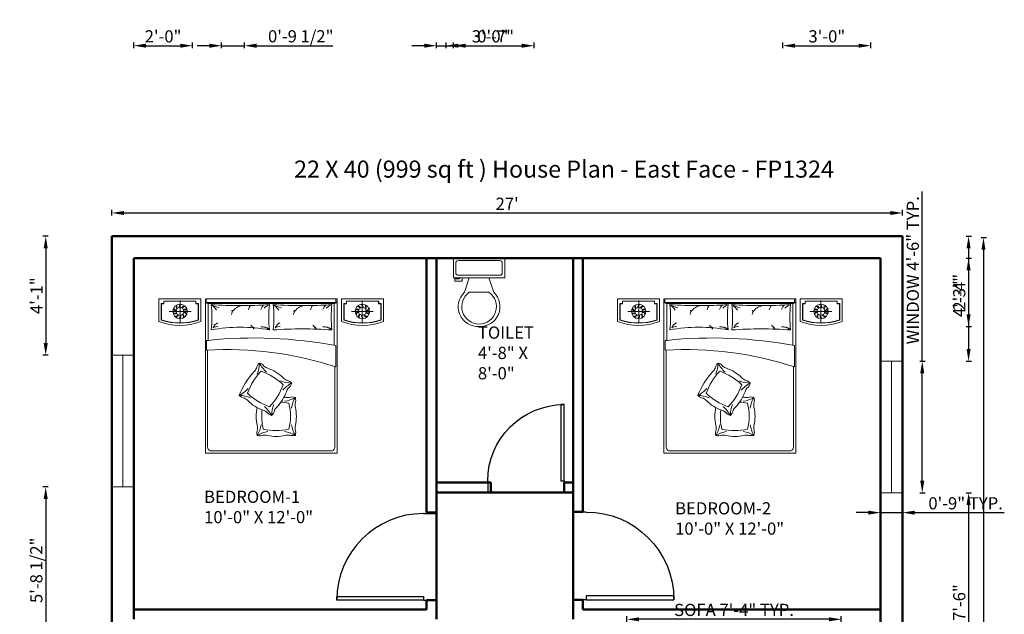
# Model space of a CAD drawing. Units: inches. Extents: x -8 to 396, y -471 to 106.
# Tile 4 of 4: x -8 to 396, y -138 to 106. Entities that reach past the tile are written whole.
import ezdxf

# ---------------------------------------------------------------- set-up
doc = ezdxf.new("R2010")
doc.units = ezdxf.units.IN
for name, color, linetype, lineweight in [('A-ANNO-DIMS', 2, 'Continuous', 18), ('A-ANNO-TEXT', 7, 'Continuous', 25), ('A-AREA-IDEN', 7, 'Continuous', 18), ('A-DOOR', 3, 'Continuous', 25), ('A-FLOR-FIXT', 9, 'Continuous', 18), ('A-GLAZ', 4, 'Continuous', 18), ('A-WALL', 7, 'Continuous', 50), ('furn', 8, 'Continuous', 18)]:
    doc.layers.add(name, color=color, linetype=linetype, lineweight=lineweight)
doc.styles.get("Standard").update_dxf_attribs({"font": 'arial.ttf'})
doc.dimstyles.new('ISO-25', dxfattribs={"dimtxt": 5, "dimasz": 5, "dimexe": 1.25, "dimexo": 0.625, "dimtad": 1, "dimlunit": 3, "dimtxsty": 'Standard', "dimcen": 2.5, "dimadec": 0, "dimazin": 0, "dimtfac": 1, "dimtmove": 0, "dimatfit": 3, "dimfxl": 1, "dimfxlon": 1, "dimarcsym": 0})

# ---------------------------------------------------------------- blocks, each defined once
blk = doc.blocks.new('*U7')
for p, q in [((9.5, -6), (9.5, -2)), ((-8, -8.5), (-8, -8)), ((-7, -8), (-7, -9.5)), ((-4, -8), (-6, -14)), ((4, -8), (6, -14)), ((-10, -8.5), (-8, -8.5)), ((-10, -9.5), (-10, -8.5)), ((-7, -9.5), (-10, -9.5)), ((4, -14), (-4, -14))]:
    blk.add_line(p, q)
blk.add_lwpolyline([(10.5, -8), (10.5, 0), (-10.5, 0), (-10.5, -8)], close=True)
for points in [[(-9.5, -2), (-9.5, -6)], [(8.5, -1), (-8.5, -1)], [(-8.5, -7), (8.5, -7)]]:
    blk.add_lwpolyline(points)
for centre, radius, start, end in [((-8.625, -1.875), 0.8839, 81.8699, 188.1301), ((8.625, -1.875), 0.8839, 351.8699, 98.1301), ((-8.625, -6.125), 0.8839, 171.869898, 278.1301), ((8.625, -6.125), 0.8839, 261.8699, 8.1301), ((-0.4772, -19.9188), 8.0953, 133.01722, 273.38), ((0.0374, -19.8731), 7.127, 124.50543, 269.7), ((-0.0373, -19.8731), 7.127, 270.3, 55.4946), ((0.4773, -19.9188), 8.0953, 266.62, 46.9828)]:
    blk.add_arc(centre, radius, start, end)
blk = doc.blocks.new('*U5')
for p, q in [((0, 0), (0, -6)), ((40, 0), (40, -6))]:
    blk.add_line(p, q)
blk.add_lwpolyline([(0, 0), (0, 40), (1.75, 40), (1.75, 0)], close=True)
blk.add_arc((0, 0), 40, 0, 90)
blk = doc.blocks.new('*D8')
at = {"layer": 'A-ANNO-DIMS', "color": 0, "lineweight": -2, "transparency": 16777216}
for p, q in [((29.97, 25.64), (29.97, 27.89)), ((34.97, 26.64), (348.97, 26.64)), ((353.97, 25.64), (353.97, 27.89))]:
    blk.add_line(p, q, dxfattribs=at)
at = {"layer": 'A-ANNO-DIMS', "color": 0, "transparency": 16777216}
for points in [[(34.97, 27.47), (34.97, 25.81), (29.97, 26.64)], [(348.97, 27.47), (348.97, 25.81), (353.97, 26.64)]]:
    blk.add_solid(points, dxfattribs=at)
at = {"layer": 'Defpoints', "color": 0, "transparency": 16777216}
for p in [(353.97, 26.64), (29.97, 16.55), (353.97, 16.55)]:
    blk.add_point(p, dxfattribs=at)
at = {"layer": 'A-ANNO-DIMS', "color": 0, "transparency": 16777216, "insert": (191.97, 29.78), "char_height": 5, "attachment_point": 5}
blk.add_mtext("27'", dxfattribs=at)
blk = doc.blocks.new('*D9')
at = {"layer": 'A-ANNO-DIMS', "color": 0, "lineweight": -2, "transparency": 16777216}
for p, q in [((386.16, 16.55), (388.41, 16.55)), ((387.16, 11.55), (387.16, -421.87)), ((386.16, -426.87), (388.41, -426.87))]:
    blk.add_line(p, q, dxfattribs=at)
at = {"layer": 'A-ANNO-DIMS', "color": 0, "transparency": 16777216}
for points in [[(386.32, 11.55), (387.99, 11.55), (387.16, 16.55)], [(386.32, -421.87), (387.99, -421.87), (387.16, -426.87)]]:
    blk.add_solid(points, dxfattribs=at)
at = {"layer": 'Defpoints', "color": 0, "transparency": 16777216}
for p in [(353.97, 16.55), (353.97, -426.87), (387.16, -426.87)]:
    blk.add_point(p, dxfattribs=at)
at = {"layer": 'A-ANNO-DIMS', "color": 0, "transparency": 16777216, "insert": (383.98, -205.16), "char_height": 5, "attachment_point": 5, "rotation": 90}
blk.add_mtext('36\'-11.43"', dxfattribs=at)
blk = doc.blocks.new('BED-DOUBLE-WITH-NIGHTSTANDS')
for p, q in [((8.67, 53.66), (8.67, 62.66)), ((19.97, 61.4), (72.06, 61.4)), ((20.23, 61.87), (20.23, 46.28)), ((71.76, 61.87), (71.76, 44.26)), ((83.36, 53.66), (83.36, 62.65)), ((4.17, 58.16), (13.17, 58.16)), ((87.86, 58.16), (78.86, 58.16))]:
    blk.add_line(p, q)
for points in [[(0, 53.96), (0, 63.32), (17.16, 63.32), (17.16, 53.96, -0.181818)], [(21.42, 50.55, 0.058596), (21.42, 60.97, 0.036889), (45.31, 60.97, 0.052163), (45.31, 50.55, 0.093111)], [(46.86, 50.55, 0.058596), (46.86, 60.97, 0.036648), (70.91, 60.97, 0.052163), (70.91, 50.55, 0.036967)], [(92.03, 53.97), (92.03, 63.33), (74.87, 63.33), (74.87, 53.97, 0.181818)], [(19.5, 46.28), (20.23, 46.28, -0.072944), (72.49, 44.11), (72.49, 35.45, 0.092568), (19.5, 42.31)]]:
    blk.add_lwpolyline(points, format="xyb", close=True)
for points in [[(1.97, 62.39), (1.97, 61.36), (0.94, 61.36)], [(2.06, 62.39), (2.06, 61.26), (0.94, 61.26)], [(1.97, 62.39), (15.19, 62.39)], [(1.97, 62.29), (15.19, 62.29)], [(15.1, 62.39), (15.1, 61.26), (16.22, 61.26)], [(15.19, 62.39), (15.19, 61.36), (16.22, 61.36)], [(19.03, 63.33), (19.03, 0), (73, 0), (73, 63.33)], [(72.49, 63.33), (72.49, 61.87), (19.34, 61.87), (19.34, 63.33), (73, 63.33)], [(76.84, 62.39), (76.84, 61.36), (75.81, 61.36)], [(76.93, 62.39), (76.93, 61.27), (75.81, 61.27)], [(90.06, 62.39), (76.84, 62.39)], [(90.06, 62.3), (76.84, 62.3)], [(89.97, 62.39), (89.97, 61.27), (91.09, 61.27)], [(90.06, 62.39), (90.06, 61.36), (91.09, 61.36)]]:
    blk.add_lwpolyline(points)
for points in [[(16.22, 61.36), (16.22, 54.62, -0.167087), (0.94, 54.62), (0.94, 61.36)], [(16.13, 61.36), (16.13, 54.68, -0.165559), (1.03, 54.68), (1.03, 61.36)], [(75.81, 61.36), (75.81, 54.62, 0.167087), (91.09, 54.62), (91.09, 61.36)], [(75.9, 61.36), (75.9, 54.69, 0.165559), (91, 54.69), (91, 61.36)], [(19.97, 42.34), (19.97, 2.5, 0.414214), (21.53, 0.94), (70.5, 0.94, 0.414214), (72.06, 2.5), (72.06, 35.61)], [(40.22, 32.4, 0.091296), (41.17, 36.97, 0.091296), (44.05, 33.3, 0.091296)], [(36.36, 24.6, 0.111006), (45.27, 19.06, 0.119549), (50.89, 28.07, 0.107813), (42, 33.64)], [(41.95, 33.62, 0.121865), (36.36, 24.6, 0.121865)], [(46.16, 15.49, 0.159461), (47.37, 17.63, -0.076283), (48.33, 18.96, 0.115075), (52.24, 25.25, -0.076283), (53.02, 26.7, 0.159461), (54.41, 28.73)], [(49.84, 29.69, 0.091296), (54.41, 28.73, 0.091296), (50.72, 25.86, 0.091296)], [(37.49, 22.77, 0.091296), (32.92, 23.74, 0.091296), (36.61, 26.6, 0.091296)], [(42.77, 9.86, 0.111006), (53.27, 9.87, 0.119549), (53.27, 20.49, 0.033212), (50.04, 20.98)], [(51.53, 21.31, 0.091296), (55.91, 22.91, 0.091296), (54.3, 18.53, 0.091296)], [(55.91, 7.31, 0.159461), (55.8, 9.77, -0.076283), (55.91, 11.41, 0.115075), (55.91, 18.81, -0.076283), (55.8, 20.45, 0.159461), (55.91, 22.91)], [(47.11, 20.06, 0.091296), (46.16, 15.49, 0.091296), (43.28, 19.16)], [(44.7, 8.91, 0.091296), (40.31, 7.31, 0.091296), (41.93, 11.69, 0.091296)], [(54.3, 11.69, 0.091296), (55.91, 7.31, 0.091296), (51.53, 8.91)]]:
    blk.add_lwpolyline(points, format="xyb")
for centre, radius in [((8.67, 58.16), 2.94), ((83.36, 58.16), 2.94), ((8.67, 58.16), 1.59), ((83.36, 58.16), 1.59)]:
    blk.add_circle(centre, radius)
for centre, radius, start, end in [((8.93, 60.36), 1.89, 172.17, 218.4897), ((8.74, 60.32), 1.44, 160.3002, 220.538), ((10.17, 59.78), 1.89, 136.17, 182.4897), ((10, 59.86), 1.44, 124.3002, 184.538), ((19.97, 62.34), 0.936, 180, 270), ((26.97, 69.69), 10.33, 237.5379, 257.5233), ((13.61, 51.22), 12.5, 36.4935, 51.2792), ((34.89, 54.79), 5.78, 96.6849, 148.3182), ((40.74, 58.08), 4.06, 141.8174, 169.8987), ((45.87, 57.5), 4.36, 130.5354, 160.3558), ((48.59, 53.82), 7.86, 114.6457, 134.1585), ((39.05, 51.22), 12.5, 36.4935, 51.2792), ((52.41, 69.69), 10.33, 237.5379, 257.5233), ((60.33, 54.79), 5.78, 96.6849, 148.3182), ((66.18, 58.08), 4.06, 141.8174, 169.8987), ((71.31, 57.5), 4.36, 130.5354, 160.3558), ((74.03, 53.82), 7.86, 114.6457, 134.1585), ((72.06, 62.34), 0.936, 270, 0), ((82.03, 59.86), 1.44, 355.462, 55.6998), ((81.86, 59.78), 1.89, 357.5103, 43.83), ((83.28, 60.32), 1.44, 319.462, 19.6998), ((83.31, 60.44), 1.89, 321.5103, 7.83), ((6.64, 58.9), 1.44, 232.3002, 292.538), ((6.65, 59.08), 1.89, 244.17, 290.4897), ((7.58, 60.09), 1.89, 208.17, 254.4897), ((7.46, 59.95), 1.44, 196.3002, 256.538), ((6.59, 57.56), 1.44, 268.3002, 328.538), ((6.49, 57.72), 1.89, 280.17, 326.4897), ((7.34, 56.45), 1.44, 304.3002, 4.538), ((7.16, 56.53), 1.89, 316.17, 2.4897), ((10.84, 58.59), 1.89, 100.17, 146.4897), ((10.75, 58.75), 1.44, 88.3002, 148.538), ((8.59, 56), 1.44, 340.3002, 40.538), ((8.41, 55.96), 1.89, 352.17, 38.4897), ((10.68, 57.23), 1.89, 64.17, 110.4897), ((10.7, 57.42), 1.44, 52.3002, 112.538), ((9.88, 56.36), 1.44, 16.3002, 76.538), ((9.75, 56.22), 1.89, 28.17, 74.4897), ((27.39, 58.01), 2.59, 335.8927, 16.1192), ((52.83, 58.01), 2.59, 335.8927, 16.1192), ((81.33, 57.42), 1.44, 67.462, 127.6998), ((81.35, 57.23), 1.89, 69.5103, 115.83), ((82.28, 56.22), 1.89, 105.5103, 151.83), ((82.15, 56.36), 1.44, 103.462, 163.6998), ((81.28, 58.75), 1.44, 31.462, 91.6998), ((81.19, 58.59), 1.89, 33.5103, 79.83), ((83.62, 55.95), 1.89, 141.5103, 187.83), ((83.44, 56), 1.44, 139.462, 199.6998), ((84.86, 56.53), 1.89, 177.5103, 223.83), ((84.69, 56.45), 1.44, 175.462, 235.6998), ((85.53, 57.72), 1.89, 213.5103, 259.83), ((85.44, 57.56), 1.44, 211.462, 271.6998), ((85.59, 59.16), 1.89, 249.5103, 295.83), ((85.61, 58.98), 1.44, 247.462, 307.6998), ((84.78, 60.03), 1.44, 283.462, 343.6998), ((84.66, 60.17), 1.89, 285.5103, 331.83), ((25.53, 50.31), 3.47, 114.2916, 160.9896), ((28.45, 43.29), 13.02, 36.2085, 45.0849), ((50.97, 50.31), 3.47, 114.2916, 160.9896), ((53.89, 43.29), 13.02, 36.2085, 45.0849), ((23.73, 49.58), 2.37, 76.4823, 128.5563), ((38.09, 50.99), 0.874, 353.7543, 77.2187), ((42.26, 47.56), 4.26, 44.406, 96.8342), ((43.06, 49.05), 2.7, 33.6349, 90.8456), ((49.17, 49.58), 2.37, 76.4823, 128.5563), ((63.53, 50.99), 0.874, 353.7543, 77.2187), ((67.7, 47.56), 4.26, 44.406, 96.8342), ((68.5, 49.05), 2.7, 33.6349, 90.8456), ((43.84, 34.06), 3.95, 132.4658, 168.7065), ((40.13, 33.31), 3.82, 37.2937, 74.0973), ((64.54, 10.81), 34.16, 138.3818, 157.7644), ((35.14, 37.29), 5.42, 315.5854, 333.0343), ((46.4, 39.96), 5.42, 233.2983, 250.7472), ((39.41, 19.4), 16.3, 45.1307, 71.3884), ((54.69, 34.83), 5.42, 225.7718, 243.2208), ((51.59, 26.4), 3.65, 39.4726, 79.6505), ((35.83, 26.42), 3.95, 222.6522, 258.8929), ((32.63, 17.7), 5.42, 45.7718, 63.2208), ((47.9, 33.13), 16.3, 225.1307, 251.3884), ((48.11, 7.06), 16.3, 77.0576, 78.7033), ((52.92, 28.24), 5.42, 257.6988, 275.1477), ((54.75, 19.45), 3.65, 71.3996, 111.5774), ((56.19, 15.11), 16.3, 166.8711, 193.1289), ((64.23, 15.22), 22.11, 173.1956, 194.0284), ((40.92, 12.57), 5.42, 53.2983, 70.7472), ((47.68, 19.75), 4.52, 218.7754, 250.3571), ((44.12, 8.37), 3.95, 159.3666, 195.6073), ((35.03, 10.24), 5.42, 355.0387, 12.4877), ((41.36, 11.12), 3.95, 254.5791, 290.8198), ((43.26, 2.03), 5.42, 77.6988, 95.1477), ((48.06, 23.21), 16.3, 257.0576, 283.3153), ((53, 2.06), 5.42, 85.2252, 102.6741), ((54.95, 11.73), 4.52, 250.7023, 282.284)]:
    blk.add_arc(centre, radius, start, end)
blk = doc.blocks.new('WINDOW-54IN')
blk.add_line((4.5, 54), (4.5, 0))
blk.add_lwpolyline([(0, 54), (9, 54), (9, 0), (0, 0)], close=True)
blk = doc.blocks.new('*D14')
at = {"layer": 'A-ANNO-DIMS', "color": 0, "lineweight": -2, "transparency": 16777216}
for p, q in [((362.07, -34.09), (362.07, 35.43)), ((361.07, -34.09), (363.32, -34.09)), ((362.07, -83.09), (362.07, -39.09)), ((361.07, -88.09), (363.32, -88.09))]:
    blk.add_line(p, q, dxfattribs=at)
at = {"layer": 'A-ANNO-DIMS', "color": 0, "transparency": 16777216}
for points in [[(361.23, -39.09), (362.9, -39.09), (362.07, -34.09)], [(361.23, -83.09), (362.9, -83.09), (362.07, -88.09)]]:
    blk.add_solid(points, dxfattribs=at)
at = {"layer": 'Defpoints', "color": 0, "transparency": 16777216}
for p in [(353.97, -34.09), (362.07, -34.09), (353.97, -88.09)]:
    blk.add_point(p, dxfattribs=at)
at = {"layer": 'A-ANNO-DIMS', "color": 0, "transparency": 16777216, "insert": (358.85, 3.17), "char_height": 5, "attachment_point": 5, "rotation": 90}
blk.add_mtext('WINDOW 4\'-6" TYP.', dxfattribs=at)
blk = doc.blocks.new('*D15')
at = {"layer": 'A-ANNO-DIMS', "color": 0, "lineweight": -2, "transparency": 16777216}
for p, q in [((339.97, -96.19), (334.97, -96.19)), ((344.97, -95.19), (344.97, -97.44)), ((344.97, -96.19), (353.97, -96.19)), ((353.97, -95.19), (353.97, -97.44)), ((358.97, -96.19), (395.69, -96.19))]:
    blk.add_line(p, q, dxfattribs=at)
at = {"layer": 'A-ANNO-DIMS', "color": 0, "transparency": 16777216}
for points in [[(339.97, -95.36), (339.97, -97.02), (344.97, -96.19)], [(358.97, -95.36), (358.97, -97.02), (353.97, -96.19)]]:
    blk.add_solid(points, dxfattribs=at)
at = {"layer": 'Defpoints', "color": 0, "transparency": 16777216}
for p in [(344.97, -88.09), (353.97, -88.09), (353.97, -96.19)]:
    blk.add_point(p, dxfattribs=at)
at = {"layer": 'A-ANNO-DIMS', "color": 0, "transparency": 16777216, "insert": (379.83, -93.01), "char_height": 5, "attachment_point": 5}
blk.add_mtext('0\'-9" TYP.', dxfattribs=at)
blk = doc.blocks.new('*D18')
at = {"layer": 'A-ANNO-DIMS', "color": 0, "lineweight": -2, "transparency": 16777216}
for p, q in [((241.05, -140.93), (241.05, -138.68)), ((323.86, -139.93), (246.05, -139.93)), ((328.86, -140.93), (328.86, -138.68))]:
    blk.add_line(p, q, dxfattribs=at)
at = {"layer": 'A-ANNO-DIMS', "color": 0, "transparency": 16777216}
for points in [[(246.05, -139.1), (246.05, -140.76), (241.05, -139.93)], [(323.86, -139.1), (323.86, -140.76), (328.86, -139.93)]]:
    blk.add_solid(points, dxfattribs=at)
at = {"layer": 'Defpoints', "color": 0, "transparency": 16777216}
for p in [(241.05, -139.93), (241.05, -153.1), (328.86, -153.1)]:
    blk.add_point(p, dxfattribs=at)
at = {"layer": 'A-ANNO-DIMS', "color": 0, "transparency": 16777216, "insert": (284.95, -136.72), "char_height": 5, "attachment_point": 5}
blk.add_mtext('SOFA 7\'-4" TYP.', dxfattribs=at)
blk = doc.blocks.new('*D28')
at = {"layer": 'A-ANNO-DIMS', "color": 0, "lineweight": -2, "transparency": 16777216}
for p, q in [((3.88, 17.13), (1.63, 17.13)), ((2.88, 12.13), (2.88, -26.66)), ((3.88, -31.66), (1.63, -31.66))]:
    blk.add_line(p, q, dxfattribs=at)
at = {"layer": 'A-ANNO-DIMS', "color": 0, "transparency": 16777216}
for points in [[(2.04, 12.13), (3.71, 12.13), (2.88, 17.13)], [(2.04, -26.66), (3.71, -26.66), (2.88, -31.66)]]:
    blk.add_solid(points, dxfattribs=at)
at = {"layer": 'Defpoints', "color": 0, "transparency": 16777216}
for p in [(29.97, 17.13), (2.88, -31.66), (29.97, -31.66)]:
    blk.add_point(p, dxfattribs=at)
at = {"layer": 'A-ANNO-DIMS', "color": 0, "transparency": 16777216, "insert": (-0.26, -7.27), "char_height": 5, "attachment_point": 5, "rotation": 90}
blk.add_mtext('4\'-1"', dxfattribs=at)
blk = doc.blocks.new('*D29')
at = {"layer": 'A-ANNO-DIMS', "color": 0, "lineweight": -2, "transparency": 16777216}
for p, q in [((3.88, -85.66), (1.63, -85.66)), ((2.88, -90.66), (2.88, -149)), ((3.88, -154), (1.63, -154))]:
    blk.add_line(p, q, dxfattribs=at)
at = {"layer": 'A-ANNO-DIMS', "color": 0, "transparency": 16777216}
for points in [[(2.04, -90.66), (3.71, -90.66), (2.88, -85.66)], [(2.04, -149), (3.71, -149), (2.88, -154)]]:
    blk.add_solid(points, dxfattribs=at)
at = {"layer": 'Defpoints', "color": 0, "transparency": 16777216}
for p in [(29.97, -85.66), (2.88, -154), (29.97, -154)]:
    blk.add_point(p, dxfattribs=at)
at = {"layer": 'A-ANNO-DIMS', "color": 0, "transparency": 16777216, "insert": (-0.33, -119.83), "char_height": 5, "attachment_point": 5, "rotation": 90}
blk.add_mtext('5\'-8 1/2"', dxfattribs=at)
blk = doc.blocks.new('*D31')
at = {"layer": 'A-ANNO-DIMS', "color": 0, "lineweight": -2, "transparency": 16777216}
for p, q in [((380.06, 17.13), (382.31, 17.13)), ((381.06, 12.13), (381.06, -29.09)), ((380.06, -34.09), (382.31, -34.09))]:
    blk.add_line(p, q, dxfattribs=at)
at = {"layer": 'A-ANNO-DIMS', "color": 0, "transparency": 16777216}
for points in [[(380.22, 12.13), (381.89, 12.13), (381.06, 17.13)], [(380.22, -29.09), (381.89, -29.09), (381.06, -34.09)]]:
    blk.add_solid(points, dxfattribs=at)
at = {"layer": 'Defpoints', "color": 0, "transparency": 16777216}
for p in [(353.97, 17.13), (353.97, -34.09), (381.06, -34.09)]:
    blk.add_point(p, dxfattribs=at)
at = {"layer": 'A-ANNO-DIMS', "color": 0, "transparency": 16777216, "insert": (377.88, -8.48), "char_height": 5, "attachment_point": 5, "rotation": 90}
blk.add_mtext('4\'-3"', dxfattribs=at)
blk = doc.blocks.new('*D32')
at = {"layer": 'A-ANNO-DIMS', "color": 0, "lineweight": -2, "transparency": 16777216}
for p, q in [((380.06, -88.09), (382.31, -88.09)), ((381.06, -93.09), (381.06, -173.04)), ((380.06, -178.04), (382.31, -178.04))]:
    blk.add_line(p, q, dxfattribs=at)
at = {"layer": 'A-ANNO-DIMS', "color": 0, "transparency": 16777216}
for points in [[(380.22, -93.09), (381.89, -93.09), (381.06, -88.09)], [(380.22, -173.04), (381.89, -173.04), (381.06, -178.04)]]:
    blk.add_solid(points, dxfattribs=at)
at = {"layer": 'Defpoints', "color": 0, "transparency": 16777216}
for p in [(353.97, -88.09), (353.97, -178.04), (381.06, -178.04)]:
    blk.add_point(p, dxfattribs=at)
at = {"layer": 'A-ANNO-DIMS', "color": 0, "transparency": 16777216, "insert": (377.88, -133.06), "char_height": 5, "attachment_point": 5, "rotation": 90}
blk.add_mtext('7\'-6"', dxfattribs=at)
blk = doc.blocks.new('*D39')
at = {"layer": 'A-ANNO-DIMS', "color": 0, "lineweight": -2, "transparency": 16777216}
for p, q in [((69.97, 95.22), (64.97, 95.22)), ((74.97, 94.22), (74.97, 96.47)), ((74.97, 95.22), (84.3, 95.22)), ((84.3, 94.22), (84.3, 96.47)), ((89.3, 95.22), (120.49, 95.22))]:
    blk.add_line(p, q, dxfattribs=at)
at = {"layer": 'A-ANNO-DIMS', "color": 0, "transparency": 16777216}
for points in [[(69.97, 96.05), (69.97, 94.38), (74.97, 95.22)], [(89.3, 96.05), (89.3, 94.38), (84.3, 95.22)]]:
    blk.add_solid(points, dxfattribs=at)
at = {"layer": 'Defpoints', "color": 0, "transparency": 16777216}
for p in [(84.3, 95.22), (74.97, -139.87), (84.3, -139.87)]:
    blk.add_point(p, dxfattribs=at)
at = {"layer": 'A-ANNO-DIMS', "color": 0, "transparency": 16777216, "insert": (107.39, 98.43), "char_height": 5, "attachment_point": 5}
blk.add_mtext('0\'-9 1/2"', dxfattribs=at)
blk = doc.blocks.new('*D40')
at = {"layer": 'A-ANNO-DIMS', "color": 0, "lineweight": -2, "transparency": 16777216}
for p, q in [((38.97, 94.22), (38.97, 96.47)), ((43.97, 95.22), (57.97, 95.22)), ((62.97, 94.22), (62.97, 96.47))]:
    blk.add_line(p, q, dxfattribs=at)
at = {"layer": 'A-ANNO-DIMS', "color": 0, "transparency": 16777216}
for points in [[(43.97, 96.05), (43.97, 94.38), (38.97, 95.22)], [(57.97, 96.05), (57.97, 94.38), (62.97, 95.22)]]:
    blk.add_solid(points, dxfattribs=at)
at = {"layer": 'Defpoints', "color": 0, "transparency": 16777216}
for p in [(62.97, 95.22), (38.97, -303.72), (62.97, -303.72)]:
    blk.add_point(p, dxfattribs=at)
at = {"layer": 'A-ANNO-DIMS', "color": 0, "transparency": 16777216, "insert": (50.97, 98.39), "char_height": 5, "attachment_point": 5}
blk.add_mtext('2\'-0"', dxfattribs=at)
blk = doc.blocks.new('*D46')
at = {"layer": 'A-ANNO-DIMS', "color": 0, "lineweight": -2, "transparency": 16777216}
for p, q in [((185.28, -452.96), (185.28, -455.21)), ((190.28, -453.96), (210.28, -453.96)), ((215.28, -452.96), (215.28, -455.21))]:
    blk.add_line(p, q, dxfattribs=at)
at = {"layer": 'A-ANNO-DIMS', "color": 0, "transparency": 16777216}
for points in [[(190.28, -453.13), (190.28, -454.8), (185.28, -453.96)], [(210.28, -453.13), (210.28, -454.8), (215.28, -453.96)]]:
    blk.add_solid(points, dxfattribs=at)
at = {"layer": 'Defpoints', "color": 0, "transparency": 16777216}
for p in [(185.28, -87.87), (215.28, -87.87), (215.28, -453.96)]:
    blk.add_point(p, dxfattribs=at)
at = {"layer": 'A-ANNO-DIMS', "color": 0, "transparency": 16777216, "insert": (200.28, -450.79), "char_height": 5, "attachment_point": 5}
blk.add_mtext('2\'-6"', dxfattribs=at)
blk = doc.blocks.new('*D47')
at = {"layer": 'A-ANNO-DIMS', "color": 0, "lineweight": -2, "transparency": 16777216}
for p, q in [((157.97, 95.22), (152.97, 95.22)), ((162.97, 94.22), (162.97, 96.47)), ((162.97, 95.22), (169.97, 95.22)), ((169.97, 94.22), (169.97, 96.47)), ((174.97, 95.22), (194.51, 95.22))]:
    blk.add_line(p, q, dxfattribs=at)
at = {"layer": 'A-ANNO-DIMS', "color": 0, "transparency": 16777216}
for points in [[(157.97, 96.05), (157.97, 94.38), (162.97, 95.22)], [(174.97, 96.05), (174.97, 94.38), (169.97, 95.22)]]:
    blk.add_solid(points, dxfattribs=at)
at = {"layer": 'Defpoints', "color": 0, "transparency": 16777216}
for p in [(169.97, 95.22), (162.97, 8.13), (169.97, 8.13)]:
    blk.add_point(p, dxfattribs=at)
at = {"layer": 'A-ANNO-DIMS', "color": 0, "transparency": 16777216, "insert": (187.24, 98.39), "char_height": 5, "attachment_point": 5}
blk.add_mtext('0\'-7"', dxfattribs=at)
blk = doc.blocks.new('*D48')
at = {"layer": 'A-ANNO-DIMS', "color": 0, "lineweight": -2, "transparency": 16777216}
for p, q in [((169.97, -452.96), (169.97, -455.21)), ((174.97, -453.96), (185.97, -453.96)), ((190.97, -452.96), (190.97, -455.21))]:
    blk.add_line(p, q, dxfattribs=at)
at = {"layer": 'A-ANNO-DIMS', "color": 0, "transparency": 16777216}
for points in [[(174.97, -453.13), (174.97, -454.8), (169.97, -453.96)], [(185.97, -453.13), (185.97, -454.8), (190.97, -453.96)]]:
    blk.add_solid(points, dxfattribs=at)
at = {"layer": 'Defpoints', "color": 0, "transparency": 16777216}
for p in [(169.97, 0.13), (190.97, 0.13), (190.97, -453.96)]:
    blk.add_point(p, dxfattribs=at)
at = {"layer": 'A-ANNO-DIMS', "color": 0, "transparency": 16777216, "insert": (180.47, -450.79), "char_height": 5, "attachment_point": 5}
blk.add_mtext('1\'-9"', dxfattribs=at)
blk = doc.blocks.new('*D49')
at = {"layer": 'A-ANNO-DIMS', "color": 0, "lineweight": -2, "transparency": 16777216}
for p, q in [((380.06, 8.13), (382.31, 8.13)), ((381.06, 3.13), (381.06, -14.87)), ((380.06, -19.87), (382.31, -19.87))]:
    blk.add_line(p, q, dxfattribs=at)
at = {"layer": 'A-ANNO-DIMS', "color": 0, "transparency": 16777216}
for points in [[(380.22, 3.13), (381.89, 3.13), (381.06, 8.13)], [(380.22, -14.87), (381.89, -14.87), (381.06, -19.87)]]:
    blk.add_solid(points, dxfattribs=at)
at = {"layer": 'Defpoints', "color": 0, "transparency": 16777216}
for p in [(190.97, 8.13), (180.47, -19.87), (381.06, -19.87)]:
    blk.add_point(p, dxfattribs=at)
at = {"layer": 'A-ANNO-DIMS', "color": 0, "transparency": 16777216, "insert": (377.92, -5.87), "char_height": 5, "attachment_point": 5, "rotation": 90}
blk.add_mtext('2\'-4"', dxfattribs=at)
blk = doc.blocks.new('*D50')
at = {"layer": 'A-ANNO-DIMS', "color": 0, "lineweight": -2, "transparency": 16777216}
for p, q in [((166.97, 94.22), (166.97, 96.47)), ((171.97, 95.22), (197.97, 95.22)), ((202.97, 94.22), (202.97, 96.47))]:
    blk.add_line(p, q, dxfattribs=at)
at = {"layer": 'A-ANNO-DIMS', "color": 0, "transparency": 16777216}
for points in [[(171.97, 96.05), (171.97, 94.38), (166.97, 95.22)], [(197.97, 96.05), (197.97, 94.38), (202.97, 95.22)]]:
    blk.add_solid(points, dxfattribs=at)
at = {"layer": 'Defpoints', "color": 0, "transparency": 16777216}
for p in [(202.97, 95.22), (166.97, -317.87), (202.97, -317.87)]:
    blk.add_point(p, dxfattribs=at)
at = {"layer": 'A-ANNO-DIMS', "color": 0, "transparency": 16777216, "insert": (184.97, 98.4), "char_height": 5, "attachment_point": 5}
blk.add_mtext('3\'-0"', dxfattribs=at)
blk = doc.blocks.new('*D52')
at = {"layer": 'A-ANNO-DIMS', "color": 0, "lineweight": -2, "transparency": 16777216}
for p, q in [((304.97, 94.22), (304.97, 96.47)), ((309.97, 95.22), (335.97, 95.22)), ((340.97, 94.22), (340.97, 96.47))]:
    blk.add_line(p, q, dxfattribs=at)
at = {"layer": 'A-ANNO-DIMS', "color": 0, "transparency": 16777216}
for points in [[(309.97, 96.05), (309.97, 94.38), (304.97, 95.22)], [(335.97, 96.05), (335.97, 94.38), (340.97, 95.22)]]:
    blk.add_solid(points, dxfattribs=at)
at = {"layer": 'Defpoints', "color": 0, "transparency": 16777216}
for p in [(340.97, 95.22), (304.97, -293.87), (340.97, -293.87)]:
    blk.add_point(p, dxfattribs=at)
at = {"layer": 'A-ANNO-DIMS', "color": 0, "transparency": 16777216, "insert": (322.97, 98.4), "char_height": 5, "attachment_point": 5}
blk.add_mtext('3\'-0"', dxfattribs=at)

msp = doc.modelspace()

# ---------------------------------------------------------------- linework, layer by layer
at = {"layer": 'A-WALL'}
for p, q in [((29.966, 17.126), (353.966, 17.126)), ((29.966, -426.874), (29.966, 17.126)), ((353.966, 17.126), (353.966, -426.874)), ((38.966, 8.126), (162.966, 8.126)), ((38.966, -139.874), (38.966, 8.126)), ((158.966, -96.08), (158.966, 8.126)), ((162.966, 8.126), (218.966, 8.126)), ((162.966, -139.874), (162.966, 8.126)), ((218.966, 8.126), (344.966, 8.126)), ((218.966, -139.874), (218.966, 8.126)), ((222.966, -95.874), (222.966, 8.126)), ((344.966, 8.126), (344.966, -417.874)), ((162.966, -83.874), (185.282, -83.874)), ((185.282, -83.874), (185.282, -87.874)), ((215.282, -83.874), (215.282, -87.874)), ((215.282, -83.874), (218.966, -83.874)), ((162.966, -87.874), (218.966, -87.874)), ((158.966, -96.08), (162.966, -96.08)), ((222.966, -95.874), (218.966, -95.874)), ((158.966, -132.08), (162.966, -132.08)), ((158.966, -135.874), (158.966, -132.08)), ((222.966, -131.874), (218.966, -131.874)), ((222.966, -135.874), (222.966, -131.874)), ((38.966, -135.874), (158.966, -135.874)), ((222.966, -135.874), (344.966, -135.874))]:
    msp.add_line(p, q, dxfattribs=at)

# ---------------------------------------------------------------- block references
at = {"layer": 'A-DOOR', "xscale": -0.7819833272519193, "yscale": 0.7819833272519193, "zscale": 0.7819833272519193}
msp.add_blockref('*U5', (215.282, -83.182), dxfattribs=at)
at = {"layer": 'A-DOOR'}
for p, xscale, yscale, zscale, rotation in [((157.639, -132.08), 0.8877503757117265, 0.8877503757117265, 0.8877503757117265, 90), ((224.356, -131.874), -0.8984837037046304, 0.8984837037046304, 0.8984837037046304, 270)]:
    msp.add_blockref('*U5', p, dxfattribs=dict(at, xscale=xscale, yscale=yscale, zscale=zscale, rotation=rotation))
at = {"layer": 'A-FLOR-FIXT'}
msp.add_blockref('*U7', (180.466, 8.126), dxfattribs=at)
at = {"layer": 'A-GLAZ'}
for p in [(29.966, -85.659), (344.966, -88.091)]:
    msp.add_blockref('WINDOW-54IN', p, dxfattribs=at)
at = {"layer": 'furn'}
for p in [(49.255, -71.857), (237.207, -71.857)]:
    msp.add_blockref('BED-DOUBLE-WITH-NIGHTSTANDS', p, dxfattribs=at)

# ---------------------------------------------------------------- texts
at = {"layer": 'A-ANNO-TEXT', "insert": (104.662, 48.134), "char_height": 7, "attachment_point": 1}
msp.add_mtext_dynamic_manual_height_columns('22 X 40 (999 sq ft ) House Plan - East Face - FP1324', width=277.00832, gutter_width=12.5, heights=[0], dxfattribs=at)
at = {"layer": 'A-AREA-IDEN', "char_height": 5, "attachment_point": 1}
for s, width, insert in [('TOILET\\P4\'-8" X 8\'-0"', 33.92558, (179.988, -19.888)), ('BEDROOM-1\\P10\'-0" X 12\'-0"', 67.54976, (67.779, -87.2)), ('BEDROOM-2\\P10\'-0" X 12\'-0"', 62.93055, (260.798, -91.915))]:
    msp.add_mtext_dynamic_manual_height_columns(s, width=width, gutter_width=12.5, heights=[0], dxfattribs=dict(at, insert=insert))

# ---------------------------------------------------------------- dimensions: what is measured, and where the dimension line sits
at = {"layer": 'A-ANNO-DIMS'}
for base, p1, p2, override, picture, middle in [((84.299, 95.216), (74.966, -139.874), (84.299, -139.874), {"dimdec": 1, "dimlfac": 1, "dimrnd": 0, "dimzin": 1, "dimdsep": 46, "dimlunit": 4, "dimfrac": 2}, '*D39', (107.395, 98.426)), ((62.966, 95.216), (38.966, -303.723), (62.966, -303.723), {"dimdec": 1, "dimlfac": 1, "dimrnd": 0, "dimzin": 1, "dimdsep": 46, "dimlunit": 4, "dimfrac": 2}, '*D40', (50.966, 98.394)), ((169.966, 95.216), (162.966, 8.126), (169.966, 8.126), {"dimdec": 1, "dimlfac": 1, "dimrnd": 0, "dimzin": 1, "dimdsep": 46, "dimlunit": 4, "dimfrac": 2}, '*D47', (187.236, 98.394)), ((202.966, 95.216), (166.966, -317.874), (202.966, -317.874), {"dimdec": 1, "dimlfac": 1, "dimrnd": 0, "dimzin": 1, "dimdsep": 46, "dimlunit": 4, "dimfrac": 2}, '*D50', (184.966, 98.396)), ((340.966, 95.216), (304.966, -293.874), (340.966, -293.874), {"dimdec": 1, "dimlfac": 1, "dimrnd": 0, "dimzin": 1, "dimdsep": 46, "dimlunit": 4, "dimfrac": 2}, '*D52', (322.966, 98.396)), ((353.966, 26.64), (29.966, 16.551), (353.966, 16.551), {"dimclrd": 0, "dimclre": 0, "dimclrt": 0}, '*D8', (191.966, 29.775)), ((190.966, -453.964), (169.966, 0.126), (190.966, 0.126), {"dimdec": 1, "dimlfac": 1, "dimrnd": 0, "dimzin": 1, "dimdsep": 46, "dimlunit": 4, "dimfrac": 2}, '*D48', (180.466, -450.786)), ((215.282, -453.964), (185.282, -87.874), (215.282, -87.874), {"dimdec": 1, "dimlfac": 1, "dimrnd": 0, "dimzin": 1, "dimdsep": 46, "dimlunit": 4, "dimfrac": 2}, '*D46', (200.282, -450.786))]:
    dim = msp.add_linear_dim(base=base, p1=p1, p2=p2, dimstyle='ISO-25', override=override, dxfattribs=at)
    dim.commit()
    dim.dimension.update_dxf_attribs({"geometry": picture, "text_midpoint": middle})
for base, p1, p2, angle, text, picture, middle in [((362.066, -34.09), (353.966, -88.09), (353.966, -34.09), 90, 'WINDOW <> TYP.', '*D14', (358.854, 3.17)), ((241.049, -139.93), (328.86, -153.102), (241.049, -153.102), 180, 'SOFA <> TYP.', '*D18', (284.954, -136.718))]:
    dim = msp.add_linear_dim(base=base, p1=p1, p2=p2, angle=angle, text=text, dimstyle='ISO-25', override={"dimdec": 1, "dimlfac": 1, "dimrnd": 0, "dimzin": 1, "dimdsep": 46, "dimlunit": 4, "dimfrac": 2}, dxfattribs=at)
    dim.commit()
    dim.dimension.update_dxf_attribs({"geometry": picture, "text_midpoint": middle})
for base, p1, p2, override, picture, middle in [((2.876, -31.659), (29.966, 17.126), (29.966, -31.659), {"dimdec": 1, "dimlfac": 1, "dimrnd": 0, "dimzin": 1, "dimdsep": 46, "dimlunit": 4, "dimfrac": 2}, '*D28', (-0.26, -7.266)), ((381.056, -34.09), (353.966, 17.126), (353.966, -34.09), {"dimdec": 1, "dimlfac": 1, "dimrnd": 0, "dimzin": 1, "dimdsep": 46, "dimlunit": 4, "dimfrac": 2}, '*D31', (377.876, -8.482)), ((387.1551, -426.874), (353.9656, 16.5511), (353.9656, -426.874), {"dimclrd": 0, "dimclre": 0, "dimclrt": 0}, '*D9', (383.9755, -205.1614)), ((381.056, -19.874), (190.966, 8.126), (180.466, -19.874), {"dimdec": 1, "dimlfac": 1, "dimrnd": 0, "dimzin": 1, "dimdsep": 46, "dimlunit": 4, "dimfrac": 2}, '*D49', (377.92, -5.874)), ((2.876, -153.998), (29.966, -85.659), (29.966, -153.998), {"dimdec": 1, "dimlfac": 1, "dimrnd": 0, "dimzin": 1, "dimdsep": 46, "dimlunit": 4, "dimfrac": 2}, '*D29', (-0.335, -119.828)), ((381.056, -178.037), (353.966, -88.09), (353.966, -178.037), {"dimdec": 1, "dimlfac": 1, "dimrnd": 0, "dimzin": 1, "dimdsep": 46, "dimlunit": 4, "dimfrac": 2}, '*D32', (377.878, -133.064))]:
    dim = msp.add_linear_dim(base=base, p1=p1, p2=p2, angle=90, dimstyle='ISO-25', override=override, dxfattribs=at)
    dim.commit()
    dim.dimension.update_dxf_attribs({"geometry": picture, "text_midpoint": middle})
dim = msp.add_linear_dim(base=(353.966, -96.19), p1=(344.966, -88.09), p2=(353.966, -88.09), text='<> TYP.', dimstyle='ISO-25', override={"dimdec": 1, "dimlfac": 1, "dimrnd": 0, "dimzin": 1, "dimdsep": 46, "dimlunit": 4, "dimfrac": 2}, dxfattribs=at)
dim.commit()
dim.dimension.update_dxf_attribs({"geometry": '*D15', "text_midpoint": (379.829, -93.013)})

doc.saveas('drawing.dxf')
